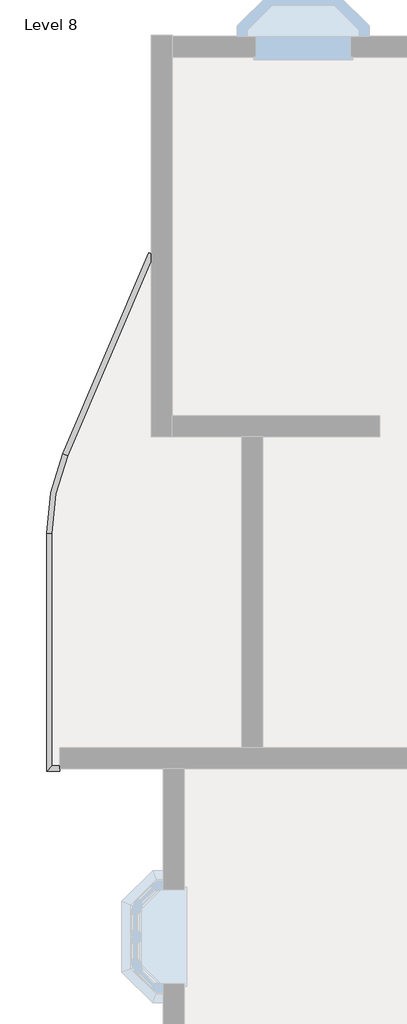
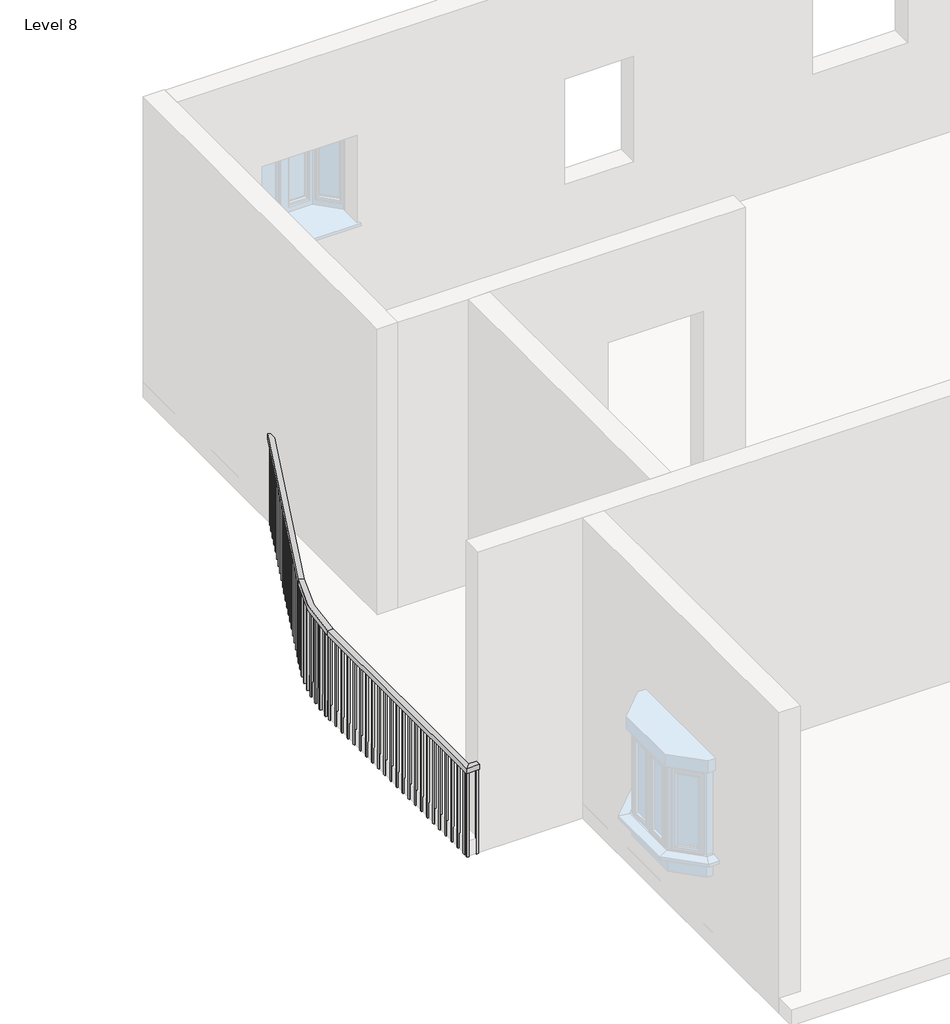
# One storey, part 7 of 14: 1 railing.
"""IFC4 building model written with IfcOpenShell, lengths in millimetres."""

from ifc_helpers import new_model, si_unit, frame, origin, place, context, project, spatial, polyline, circle_curve, outline, extrude, element, save
from ifc_brep_helpers import plane_surface, cylinder_surface, revolved_surface, advanced_brep

model = new_model("IFC4")

# Units and contexts
model_context = context("Model", 3, world=origin())
ifc_project = project(units=[si_unit("LENGTHUNIT", "METRE", prefix="MILLI")], contexts=[model_context])

# Site, building, storey
site = spatial("IfcSite", under=ifc_project)
building = spatial("IfcBuilding", under=site)
storey = spatial("IfcBuildingStorey", under=building, Name="Level 8", Elevation=21336.0)

# Railing
placement = place(None, origin())
element("IfcRailing", 1, ObjectType="Handrail - Rectangular", at=placement, inside=storey, context=model_context, shape_type="SolidModel", body=[
    advanced_brep(
    [(-12381.4379579, -2441.2590879, 22250.4), (-12381.4379579, -2441.2590879, 22199.6), (-12428.1364721, -2421.2618688, 22199.6), (-12428.1364721, -2421.2618688, 22250.4), (-13216.1814979, -4390.5942894, 22250.4), (-13216.1814979, -4390.5942894, 22199.6), (-13262.8800121, -4370.5970703, 22199.6), (-13262.8800121, -4370.5970703, 22250.4), (-13369.987215, -5140.4900045, 22199.6), (-13369.987215, -5140.4900045, 22250.4), (-13420.787215, -5140.4900045, 22199.6), (-13420.787215, -5140.4900045, 22250.4), (-13369.987215, -7396.5416506, 22250.4), (-13369.987215, -7396.5416506, 22199.6), (-13420.787215, -7447.3416506, 22199.6), (-13420.787215, -7447.3416506, 22250.4), (-13293.787215, -7396.5416506, 22250.4), (-13293.787215, -7447.3416506, 22250.4), (-13293.787215, -7447.3416506, 22199.6), (-13293.787215, -7396.5416506, 22199.6)],
    [
        (0, 1),
        (1, 2),
        (2, 3),
        (3, 0),
        (0, 4),
        (4, 5),
        (5, 1),
        (5, 6),
        (6, 2),
        (6, 7),
        (7, 3),
        (7, 4),
        (8, 5, circle_curve(frame((-11464.987215, -5140.4900045, 22199.6), z_axis=(0.0, 0.0, -1.0), x_axis=(-0.9192620907623801, 0.39364604467361003, 0.0)), 1905.0)),
        (4, 9, circle_curve(frame((-11464.987215, -5140.4900045, 22250.4), z_axis=(0.0, 0.0, 1.0), x_axis=(-0.9192620907623801, 0.39364604467361003, 0.0)), 1905.0)),
        (9, 8),
        (10, 6, circle_curve(frame((-11464.987215, -5140.4900045, 22199.6), z_axis=(0.0, 0.0, -1.0), x_axis=(-0.9192620907623801, 0.39364604467361003, 0.0)), 1955.8)),
        (8, 10),
        (11, 7, circle_curve(frame((-11464.987215, -5140.4900045, 22250.4), z_axis=(0.0, 0.0, -1.0), x_axis=(-0.9192620907623801, 0.39364604467361003, 0.0)), 1955.8)),
        (10, 11),
        (11, 9),
        (9, 12),
        (12, 13),
        (13, 8),
        (13, 14),
        (14, 10),
        (14, 15),
        (15, 11),
        (15, 12),
        (16, 17),
        (17, 18),
        (18, 19),
        (19, 16),
        (12, 16),
        (19, 13),
        (18, 14),
        (17, 15),
    ],
    [
        plane_surface(frame((-12404.787215, -2431.2604783, 22250.4), z_axis=(0.39364604467361003, 0.9192620907623801, 0.0), x_axis=(0.9192620907623801, -0.39364604467361003, 0.0))),
        plane_surface(frame((-12381.4379579, -2441.2590879, 22250.4), z_axis=(0.91926209076238, -0.39364604467361014, 0.0), x_axis=(-0.39364604467361014, -0.91926209076238, 0.0))),
        plane_surface(frame((-12381.4379579, -2441.2590879, 22199.6), z_axis=(0.0, 0.0, -1.0), x_axis=(-0.39364604467361014, -0.91926209076238, 0.0))),
        plane_surface(frame((-12428.1364721, -2421.2618688, 22199.6), z_axis=(-0.91926209076238, 0.39364604467361014, 0.0), x_axis=(-0.39364604467361014, -0.91926209076238, 0.0))),
        plane_surface(frame((-12428.1364721, -2421.2618688, 22250.4), z_axis=(0.0, 0.0, 1.0), x_axis=(-0.39364604467361014, -0.91926209076238, 0.0))),
        revolved_surface(polyline([(-13216.181497902333, -4390.594289396773, 22250.4), (-13216.181497902333, -4390.594289396773, 22199.6)]), (-11464.987215, -5140.4900045, 22250.4), (0.0, 0.0, 1.0)),
        plane_surface(frame((-11464.987215, -5140.4900045, 22199.6), z_axis=(0.0, 0.0, -1.0000000000000002), x_axis=(-0.9192620907623801, 0.39364604467361003, 0.0))),
        cylinder_surface(frame((-11464.987215, -5140.4900045, 22250.4), z_axis=(0.0, 0.0, 1.0), x_axis=(-0.9192620907623801, 0.39364604467361003, 0.0)), 1955.8),
        plane_surface(frame((-11464.987215, -5140.4900045, 22250.4), z_axis=(0.0, 0.0, 1.0000000000000002), x_axis=(-0.9192620907623801, 0.39364604467361003, 0.0))),
        plane_surface(frame((-13369.987215, -5140.4900045, 22250.4), z_axis=(1.0, 0.0, 0.0), x_axis=(0.0, -1.0, 0.0))),
        plane_surface(frame((-13369.987215, -5140.4900045, 22199.6), z_axis=(0.0, 0.0, -1.0), x_axis=(0.0, -1.0, 0.0))),
        plane_surface(frame((-13420.787215, -5140.4900045, 22199.6), z_axis=(-1.0, 0.0, 0.0), x_axis=(0.0, -1.0, 0.0))),
        plane_surface(frame((-13420.787215, -5140.4900045, 22250.4), z_axis=(0.0, 0.0, 1.0), x_axis=(0.0, -1.0, 0.0))),
        plane_surface(frame((-13293.787215, -7421.9416506, 22250.4), z_axis=(1.0, 0.0, 0.0), x_axis=(0.0, 1.0, 0.0))),
        plane_surface(frame((-13369.987215, -7396.5416506, 22250.4), z_axis=(0.0, 1.0, 0.0), x_axis=(1.0, 0.0, 0.0))),
        plane_surface(frame((-13369.987215, -7396.5416506, 22199.6), z_axis=(0.0, 0.0, -1.0), x_axis=(1.0, 0.0, 0.0))),
        plane_surface(frame((-13420.787215, -7447.3416506, 22199.6), z_axis=(0.0, -1.0, 0.0), x_axis=(1.0, 0.0, 0.0))),
        plane_surface(frame((-13420.787215, -7447.3416506, 22250.4), z_axis=(0.0, 0.0, 1.0), x_axis=(1.0, 0.0, 0.0))),
    ],
    [
        (0, [[1, 2, 3, 4]]),
        (1, [[-1, 5, 6, 7]]),
        (2, [[-2, -7, 8, 9]]),
        (3, [[-3, -9, 10, 11]]),
        (4, [[-4, -11, 12, -5]]),
        (5, [[13, -6, 14, 15]]),
        (6, [[16, -8, -13, 17]]),
        (7, [[18, -10, -16, 19]]),
        (8, [[-14, -12, -18, 20]]),
        (9, [[-15, 21, 22, 23]]),
        (10, [[-17, -23, 24, 25]]),
        (11, [[-19, -25, 26, 27]]),
        (12, [[-20, -27, 28, -21]]),
        (13, [[29, 30, 31, 32]]),
        (14, [[-22, 33, -32, 34]]),
        (15, [[-24, -34, -31, 35]]),
        (16, [[-26, -35, -30, 36]]),
        (17, [[-28, -36, -29, -33]]),
    ],
),
    extrude(outline(polyline([(-13404.912215, -7366.1650045), (-13385.862215, -7366.1650045), (-13385.862215, -7385.2150045), (-13404.912215, -7385.2150045), (-13404.912215, -7366.1650045)])), frame((0.0, 0.0, 21336.0), z_axis=(0.0, 0.0, 1.0), x_axis=(1.0, 0.0, 0.0)), (0.0, 0.0, 1.0), 863.6),
    extrude(outline(polyline([(-13404.912215, -7264.5650045), (-13385.862215, -7264.5650045), (-13385.862215, -7283.6150045), (-13404.912215, -7283.6150045), (-13404.912215, -7264.5650045)])), frame((0.0, 0.0, 21336.0), z_axis=(0.0, 0.0, 1.0), x_axis=(1.0, 0.0, 0.0)), (0.0, 0.0, 1.0), 863.6),
    extrude(outline(polyline([(-13404.912215, -7162.9650045), (-13385.862215, -7162.9650045), (-13385.862215, -7182.0150045), (-13404.912215, -7182.0150045), (-13404.912215, -7162.9650045)])), frame((0.0, 0.0, 21336.0), z_axis=(0.0, 0.0, 1.0), x_axis=(1.0, 0.0, 0.0)), (0.0, 0.0, 1.0), 863.6),
    extrude(outline(polyline([(-13404.912215, -7061.3650045), (-13385.862215, -7061.3650045), (-13385.862215, -7080.4150045), (-13404.912215, -7080.4150045), (-13404.912215, -7061.3650045)])), frame((0.0, 0.0, 21336.0), z_axis=(0.0, 0.0, 1.0), x_axis=(1.0, 0.0, 0.0)), (0.0, 0.0, 1.0), 863.6),
    extrude(outline(polyline([(-13404.912215, -6959.7650045), (-13385.862215, -6959.7650045), (-13385.862215, -6978.8150045), (-13404.912215, -6978.8150045), (-13404.912215, -6959.7650045)])), frame((0.0, 0.0, 21336.0), z_axis=(0.0, 0.0, 1.0), x_axis=(1.0, 0.0, 0.0)), (0.0, 0.0, 1.0), 863.6),
    extrude(outline(polyline([(-13404.912215, -6858.1650045), (-13385.862215, -6858.1650045), (-13385.862215, -6877.2150045), (-13404.912215, -6877.2150045), (-13404.912215, -6858.1650045)])), frame((0.0, 0.0, 21336.0), z_axis=(0.0, 0.0, 1.0), x_axis=(1.0, 0.0, 0.0)), (0.0, 0.0, 1.0), 863.6),
    extrude(outline(polyline([(-13404.912215, -6756.5650045), (-13385.862215, -6756.5650045), (-13385.862215, -6775.6150045), (-13404.912215, -6775.6150045), (-13404.912215, -6756.5650045)])), frame((0.0, 0.0, 21336.0), z_axis=(0.0, 0.0, 1.0), x_axis=(1.0, 0.0, 0.0)), (0.0, 0.0, 1.0), 863.6),
    extrude(outline(polyline([(-13404.912215, -6654.9650045), (-13385.862215, -6654.9650045), (-13385.862215, -6674.0150045), (-13404.912215, -6674.0150045), (-13404.912215, -6654.9650045)])), frame((0.0, 0.0, 21336.0), z_axis=(0.0, 0.0, 1.0), x_axis=(1.0, 0.0, 0.0)), (0.0, 0.0, 1.0), 863.6),
    extrude(outline(polyline([(-13404.912215, -6553.3650045), (-13385.862215, -6553.3650045), (-13385.862215, -6572.4150045), (-13404.912215, -6572.4150045), (-13404.912215, -6553.3650045)])), frame((0.0, 0.0, 21336.0), z_axis=(0.0, 0.0, 1.0), x_axis=(1.0, 0.0, 0.0)), (0.0, 0.0, 1.0), 863.6),
    extrude(outline(polyline([(-13404.912215, -6451.7650045), (-13385.862215, -6451.7650045), (-13385.862215, -6470.8150045), (-13404.912215, -6470.8150045), (-13404.912215, -6451.7650045)])), frame((0.0, 0.0, 21336.0), z_axis=(0.0, 0.0, 1.0), x_axis=(1.0, 0.0, 0.0)), (0.0, 0.0, 1.0), 863.6),
    extrude(outline(polyline([(-13404.912215, -6350.1650045), (-13385.862215, -6350.1650045), (-13385.862215, -6369.2150045), (-13404.912215, -6369.2150045), (-13404.912215, -6350.1650045)])), frame((0.0, 0.0, 21336.0), z_axis=(0.0, 0.0, 1.0), x_axis=(1.0, 0.0, 0.0)), (0.0, 0.0, 1.0), 863.6),
    extrude(outline(polyline([(-13404.912215, -6248.5650045), (-13385.862215, -6248.5650045), (-13385.862215, -6267.6150045), (-13404.912215, -6267.6150045), (-13404.912215, -6248.5650045)])), frame((0.0, 0.0, 21336.0), z_axis=(0.0, 0.0, 1.0), x_axis=(1.0, 0.0, 0.0)), (0.0, 0.0, 1.0), 863.6),
    extrude(outline(polyline([(-13404.912215, -6146.9650045), (-13385.862215, -6146.9650045), (-13385.862215, -6166.0150045), (-13404.912215, -6166.0150045), (-13404.912215, -6146.9650045)])), frame((0.0, 0.0, 21336.0), z_axis=(0.0, 0.0, 1.0), x_axis=(1.0, 0.0, 0.0)), (0.0, 0.0, 1.0), 863.6),
    extrude(outline(polyline([(-13404.912215, -6045.3650045), (-13385.862215, -6045.3650045), (-13385.862215, -6064.4150045), (-13404.912215, -6064.4150045), (-13404.912215, -6045.3650045)])), frame((0.0, 0.0, 21336.0), z_axis=(0.0, 0.0, 1.0), x_axis=(1.0, 0.0, 0.0)), (0.0, 0.0, 1.0), 863.6),
    extrude(outline(polyline([(-13404.912215, -5943.7650045), (-13385.862215, -5943.7650045), (-13385.862215, -5962.8150045), (-13404.912215, -5962.8150045), (-13404.912215, -5943.7650045)])), frame((0.0, 0.0, 21336.0), z_axis=(0.0, 0.0, 1.0), x_axis=(1.0, 0.0, 0.0)), (0.0, 0.0, 1.0), 863.6),
    extrude(outline(polyline([(-13404.912215, -5842.1650045), (-13385.862215, -5842.1650045), (-13385.862215, -5861.2150045), (-13404.912215, -5861.2150045), (-13404.912215, -5842.1650045)])), frame((0.0, 0.0, 21336.0), z_axis=(0.0, 0.0, 1.0), x_axis=(1.0, 0.0, 0.0)), (0.0, 0.0, 1.0), 863.6),
    extrude(outline(polyline([(-13404.912215, -5740.5650045), (-13385.862215, -5740.5650045), (-13385.862215, -5759.6150045), (-13404.912215, -5759.6150045), (-13404.912215, -5740.5650045)])), frame((0.0, 0.0, 21336.0), z_axis=(0.0, 0.0, 1.0), x_axis=(1.0, 0.0, 0.0)), (0.0, 0.0, 1.0), 863.6),
    extrude(outline(polyline([(-13404.912215, -5638.9650045), (-13385.862215, -5638.9650045), (-13385.862215, -5658.0150045), (-13404.912215, -5658.0150045), (-13404.912215, -5638.9650045)])), frame((0.0, 0.0, 21336.0), z_axis=(0.0, 0.0, 1.0), x_axis=(1.0, 0.0, 0.0)), (0.0, 0.0, 1.0), 863.6),
    extrude(outline(polyline([(-13404.912215, -5537.3650045), (-13385.862215, -5537.3650045), (-13385.862215, -5556.4150045), (-13404.912215, -5556.4150045), (-13404.912215, -5537.3650045)])), frame((0.0, 0.0, 21336.0), z_axis=(0.0, 0.0, 1.0), x_axis=(1.0, 0.0, 0.0)), (0.0, 0.0, 1.0), 863.6),
    extrude(outline(polyline([(-13404.912215, -5435.7650045), (-13385.862215, -5435.7650045), (-13385.862215, -5454.8150045), (-13404.912215, -5454.8150045), (-13404.912215, -5435.7650045)])), frame((0.0, 0.0, 21336.0), z_axis=(0.0, 0.0, 1.0), x_axis=(1.0, 0.0, 0.0)), (0.0, 0.0, 1.0), 863.6),
    extrude(outline(polyline([(-13404.912215, -5334.1650045), (-13385.862215, -5334.1650045), (-13385.862215, -5353.2150045), (-13404.912215, -5353.2150045), (-13404.912215, -5334.1650045)])), frame((0.0, 0.0, 21336.0), z_axis=(0.0, 0.0, 1.0), x_axis=(1.0, 0.0, 0.0)), (0.0, 0.0, 1.0), 863.6),
    extrude(outline(polyline([(-13404.912215, -5232.5650045), (-13385.862215, -5232.5650045), (-13385.862215, -5251.6150045), (-13404.912215, -5251.6150045), (-13404.912215, -5232.5650045)])), frame((0.0, 0.0, 21336.0), z_axis=(0.0, 0.0, 1.0), x_axis=(1.0, 0.0, 0.0)), (0.0, 0.0, 1.0), 863.6),
    extrude(outline(polyline([(-13403.2986616, -5060.8127369), (-13384.2611239, -5061.5016911), (-13384.9500781, -5080.5392288), (-13403.9876158, -5079.8502746), (-13403.2986616, -5060.8127369)])), frame((0.0, 0.0, 21336.0), z_axis=(0.0, 0.0, 1.0), x_axis=(1.0, 0.0, 0.0)), (0.0, 0.0, 1.0), 863.6),
    extrude(outline(polyline([(-13396.4230348, -4958.9537683), (-13377.4481028, -4960.6432816), (-13379.1376161, -4979.6182136), (-13398.1125481, -4977.9287003), (-13396.4230348, -4958.9537683)])), frame((0.0, 0.0, 21336.0), z_axis=(0.0, 0.0, 1.0), x_axis=(1.0, 0.0, 0.0)), (0.0, 0.0, 1.0), 863.6),
    extrude(outline(polyline([(-13384.1984052, -4857.5975541), (-13365.3386289, -4860.2829475), (-13368.0240223, -4879.1427238), (-13386.8837986, -4876.4573304), (-13384.1984052, -4857.5975541)])), frame((0.0, 0.0, 21336.0), z_axis=(0.0, 0.0, 1.0), x_axis=(1.0, 0.0, 0.0)), (0.0, 0.0, 1.0), 863.6),
    extrude(outline(polyline([(-13366.6586282, -4757.0247946), (-13347.9662387, -4760.698631), (-13351.6400752, -4779.3910205), (-13370.3324647, -4775.7171841), (-13366.6586282, -4757.0247946)])), frame((0.0, 0.0, 21336.0), z_axis=(0.0, 0.0, 1.0), x_axis=(1.0, 0.0, 0.0)), (0.0, 0.0, 1.0), 863.6),
    extrude(outline(polyline([(-13343.8522793, -4657.5140204), (-13325.3790441, -4662.1661254), (-13330.0311492, -4680.6393606), (-13348.5043844, -4675.9872556), (-13343.8522793, -4657.5140204)])), frame((0.0, 0.0, 21336.0), z_axis=(0.0, 0.0, 1.0), x_axis=(1.0, 0.0, 0.0)), (0.0, 0.0, 1.0), 863.6),
    extrude(outline(polyline([(-13315.8425193, -4559.340821), (-13297.6395991, -4564.9583109), (-13303.257089, -4583.1612312), (-13321.4600093, -4577.5437413), (-13315.8425193, -4559.340821)])), frame((0.0, 0.0, 21336.0), z_axis=(0.0, 0.0, 1.0), x_axis=(1.0, 0.0, 0.0)), (0.0, 0.0, 1.0), 863.6),
    extrude(outline(polyline([(-13282.7069198, -4462.7770815), (-13264.8247264, -4469.344399), (-13271.3920438, -4487.2265924), (-13289.2742372, -4480.659275), (-13282.7069198, -4462.7770815)])), frame((0.0, 0.0, 21336.0), z_axis=(0.0, 0.0, 1.0), x_axis=(1.0, 0.0, 0.0)), (0.0, 0.0, 1.0), 863.6),
    extrude(outline(polyline([(-13209.6824706, -4286.6955968), (-13192.1705278, -4294.1945539), (-13199.6694849, -4311.7064967), (-13217.1814277, -4304.2075396), (-13209.6824706, -4286.6955968)])), frame((0.0, 0.0, 21336.0), z_axis=(0.0, 0.0, 1.0), x_axis=(1.0, 0.0, 0.0)), (0.0, 0.0, 1.0), 863.6),
    extrude(outline(polyline([(-13169.6880325, -4193.2985683), (-13152.1760896, -4200.7975255), (-13159.6750468, -4218.3094683), (-13177.1869896, -4210.8105112), (-13169.6880325, -4193.2985683)])), frame((0.0, 0.0, 21336.0), z_axis=(0.0, 0.0, 1.0), x_axis=(1.0, 0.0, 0.0)), (0.0, 0.0, 1.0), 863.6),
    extrude(outline(polyline([(-13129.6935943, -4099.9015399), (-13112.1816515, -4107.4004971), (-13119.6806086, -4124.9124399), (-13137.1925515, -4117.4134827), (-13129.6935943, -4099.9015399)])), frame((0.0, 0.0, 21336.0), z_axis=(0.0, 0.0, 1.0), x_axis=(1.0, 0.0, 0.0)), (0.0, 0.0, 1.0), 863.6),
    extrude(outline(polyline([(-13089.6991562, -4006.5045115), (-13072.1872133, -4014.0034686), (-13079.6861705, -4031.5154115), (-13097.1981133, -4024.0164543), (-13089.6991562, -4006.5045115)])), frame((0.0, 0.0, 21336.0), z_axis=(0.0, 0.0, 1.0), x_axis=(1.0, 0.0, 0.0)), (0.0, 0.0, 1.0), 863.6),
    extrude(outline(polyline([(-13049.704718, -3913.1074831), (-13032.1927752, -3920.6064402), (-13039.6917324, -3938.1183831), (-13057.2036752, -3930.6194259), (-13049.704718, -3913.1074831)])), frame((0.0, 0.0, 21336.0), z_axis=(0.0, 0.0, 1.0), x_axis=(1.0, 0.0, 0.0)), (0.0, 0.0, 1.0), 863.6),
    extrude(outline(polyline([(-13009.7102799, -3819.7104546), (-12992.1983371, -3827.2094118), (-12999.6972942, -3844.7213546), (-13017.209237, -3837.2223975), (-13009.7102799, -3819.7104546)])), frame((0.0, 0.0, 21336.0), z_axis=(0.0, 0.0, 1.0), x_axis=(1.0, 0.0, 0.0)), (0.0, 0.0, 1.0), 863.6),
    extrude(outline(polyline([(-12969.7158418, -3726.3134262), (-12952.2038989, -3733.8123834), (-12959.7028561, -3751.3243262), (-12977.2147989, -3743.8253691), (-12969.7158418, -3726.3134262)])), frame((0.0, 0.0, 21336.0), z_axis=(0.0, 0.0, 1.0), x_axis=(1.0, 0.0, 0.0)), (0.0, 0.0, 1.0), 863.6),
    extrude(outline(polyline([(-12929.7214036, -3632.9163978), (-12912.2094608, -3640.415355), (-12919.7084179, -3657.9272978), (-12937.2203608, -3650.4283406), (-12929.7214036, -3632.9163978)])), frame((0.0, 0.0, 21336.0), z_axis=(0.0, 0.0, 1.0), x_axis=(1.0, 0.0, 0.0)), (0.0, 0.0, 1.0), 863.6),
    extrude(outline(polyline([(-12889.7269655, -3539.5193694), (-12872.2150227, -3547.0183265), (-12879.7139798, -3564.5302694), (-12897.2259226, -3557.0313122), (-12889.7269655, -3539.5193694)])), frame((0.0, 0.0, 21336.0), z_axis=(0.0, 0.0, 1.0), x_axis=(1.0, 0.0, 0.0)), (0.0, 0.0, 1.0), 863.6),
    extrude(outline(polyline([(-12849.7325273, -3446.122341), (-12832.2205845, -3453.6212981), (-12839.7195417, -3471.1332409), (-12857.2314845, -3463.6342838), (-12849.7325273, -3446.122341)])), frame((0.0, 0.0, 21336.0), z_axis=(0.0, 0.0, 1.0), x_axis=(1.0, 0.0, 0.0)), (0.0, 0.0, 1.0), 863.6),
    extrude(outline(polyline([(-12809.7380892, -3352.7253125), (-12792.2261464, -3360.2242697), (-12799.7251035, -3377.7362125), (-12817.2370464, -3370.2372554), (-12809.7380892, -3352.7253125)])), frame((0.0, 0.0, 21336.0), z_axis=(0.0, 0.0, 1.0), x_axis=(1.0, 0.0, 0.0)), (0.0, 0.0, 1.0), 863.6),
    extrude(outline(polyline([(-12769.7436511, -3259.3282841), (-12752.2317082, -3266.8272413), (-12759.7306654, -3284.3391841), (-12777.2426082, -3276.8402269), (-12769.7436511, -3259.3282841)])), frame((0.0, 0.0, 21336.0), z_axis=(0.0, 0.0, 1.0), x_axis=(1.0, 0.0, 0.0)), (0.0, 0.0, 1.0), 863.6),
    extrude(outline(polyline([(-12729.7492129, -3165.9312557), (-12712.2372701, -3173.4302129), (-12719.7362272, -3190.9421557), (-12737.2481701, -3183.4431985), (-12729.7492129, -3165.9312557)])), frame((0.0, 0.0, 21336.0), z_axis=(0.0, 0.0, 1.0), x_axis=(1.0, 0.0, 0.0)), (0.0, 0.0, 1.0), 863.6),
    extrude(outline(polyline([(-12689.7547748, -3072.5342273), (-12672.242832, -3080.0331844), (-12679.7417891, -3097.5451273), (-12697.2537319, -3090.0461701), (-12689.7547748, -3072.5342273)])), frame((0.0, 0.0, 21336.0), z_axis=(0.0, 0.0, 1.0), x_axis=(1.0, 0.0, 0.0)), (0.0, 0.0, 1.0), 863.6),
    extrude(outline(polyline([(-12649.7603366, -2979.1371989), (-12632.2483938, -2986.636156), (-12639.747351, -3004.1480988), (-12657.2592938, -2996.6491417), (-12649.7603366, -2979.1371989)])), frame((0.0, 0.0, 21336.0), z_axis=(0.0, 0.0, 1.0), x_axis=(1.0, 0.0, 0.0)), (0.0, 0.0, 1.0), 863.6),
    extrude(outline(polyline([(-12609.7658985, -2885.7401704), (-12592.2539557, -2893.2391276), (-12599.7529128, -2910.7510704), (-12617.2648557, -2903.2521133), (-12609.7658985, -2885.7401704)])), frame((0.0, 0.0, 21336.0), z_axis=(0.0, 0.0, 1.0), x_axis=(1.0, 0.0, 0.0)), (0.0, 0.0, 1.0), 863.6),
    extrude(outline(polyline([(-12569.7714604, -2792.343142), (-12552.2595175, -2799.8420992), (-12559.7584747, -2817.354042), (-12577.2704175, -2809.8550848), (-12569.7714604, -2792.343142)])), frame((0.0, 0.0, 21336.0), z_axis=(0.0, 0.0, 1.0), x_axis=(1.0, 0.0, 0.0)), (0.0, 0.0, 1.0), 863.6),
    extrude(outline(polyline([(-12529.7770222, -2698.9461136), (-12512.2650794, -2706.4450707), (-12519.7640366, -2723.9570136), (-12537.2759794, -2716.4580564), (-12529.7770222, -2698.9461136)])), frame((0.0, 0.0, 21336.0), z_axis=(0.0, 0.0, 1.0), x_axis=(1.0, 0.0, 0.0)), (0.0, 0.0, 1.0), 863.6),
    extrude(outline(polyline([(-12489.7825841, -2605.5490852), (-12472.2706413, -2613.0480423), (-12479.7695984, -2630.5599852), (-12497.2815412, -2623.061028), (-12489.7825841, -2605.5490852)])), frame((0.0, 0.0, 21336.0), z_axis=(0.0, 0.0, 1.0), x_axis=(1.0, 0.0, 0.0)), (0.0, 0.0, 1.0), 863.6),
    extrude(outline(polyline([(-12449.788146, -2512.1520567), (-12432.2762031, -2519.6510139), (-12439.7751603, -2537.1629567), (-12457.2871031, -2529.6639996), (-12449.788146, -2512.1520567)])), frame((0.0, 0.0, 21336.0), z_axis=(0.0, 0.0, 1.0), x_axis=(1.0, 0.0, 0.0)), (0.0, 0.0, 1.0), 863.6),
    extrude(outline(polyline([(-13404.912215, -7412.4166506), (-13385.862215, -7412.4166506), (-13385.862215, -7431.4666506), (-13404.912215, -7431.4666506), (-13404.912215, -7412.4166506)])), frame((0.0, 0.0, 21336.0), z_axis=(0.0, 0.0, 1.0), x_axis=(1.0, 0.0, 0.0)), (0.0, 0.0, 1.0), 863.6),
    extrude(outline(polyline([(-13404.912215, -5130.9650045), (-13385.862215, -5130.9650045), (-13385.862215, -5150.0150045), (-13404.912215, -5150.0150045), (-13404.912215, -5130.9650045)])), frame((0.0, 0.0, 21336.0), z_axis=(0.0, 0.0, 1.0), x_axis=(1.0, 0.0, 0.0)), (0.0, 0.0, 1.0), 863.6),
    extrude(outline(polyline([(-13244.5372478, -4368.0902299), (-13227.025305, -4375.589187), (-13234.5242621, -4393.1011299), (-13252.036205, -4385.6021727), (-13244.5372478, -4368.0902299)])), frame((0.0, 0.0, 21336.0), z_axis=(0.0, 0.0, 1.0), x_axis=(1.0, 0.0, 0.0)), (0.0, 0.0, 1.0), 863.6),
    extrude(outline(polyline([(-13312.837215, -7431.4666506), (-13312.837215, -7412.4166506), (-13293.787215, -7412.4166506), (-13293.787215, -7431.4666506), (-13312.837215, -7431.4666506)])), frame((0.0, 0.0, 21336.0), z_axis=(0.0, 0.0, 1.0), x_axis=(1.0, 0.0, 0.0)), (0.0, 0.0, 1.0), 863.6),
    extrude(outline(polyline([(-12413.5431864, -2427.5109997), (-12396.0312436, -2435.0099569), (-12403.5302007, -2452.5218997), (-12421.0421435, -2445.0229426), (-12413.5431864, -2427.5109997)])), frame((0.0, 0.0, 21336.0), z_axis=(0.0, 0.0, 1.0), x_axis=(1.0, 0.0, 0.0)), (0.0, 0.0, 1.0), 863.6),
])

save(model, "model.ifc")

# Revit data of these elements
# Type "Handrail - Rectangular"
#   Assembly Code = "C2010400"
#   built-in parameter 1008612 = 0.0416667 (stored number, unit not read)
#   built-in parameter 1008611 = 0.0416667 (stored number, unit not read)
#   built-in parameter 1008609 = 0.333333 (stored number, unit not read)
#   built-in parameter 1008604 = 0.166667 (stored number, unit not read)
#   built-in parameter 1008603 = 0.166667 (stored number, unit not read)
#   Railing Height = 3' - 0"
#   built-in parameter 1008630 = 2
#   built-in parameter 1008610 = 2
#   built-in parameter 1008618 = Baluster - Square : 3/4"
# Element 1 (IfcRailing, "Handrail - Rectangular")
#   Phase Created = New Construction
